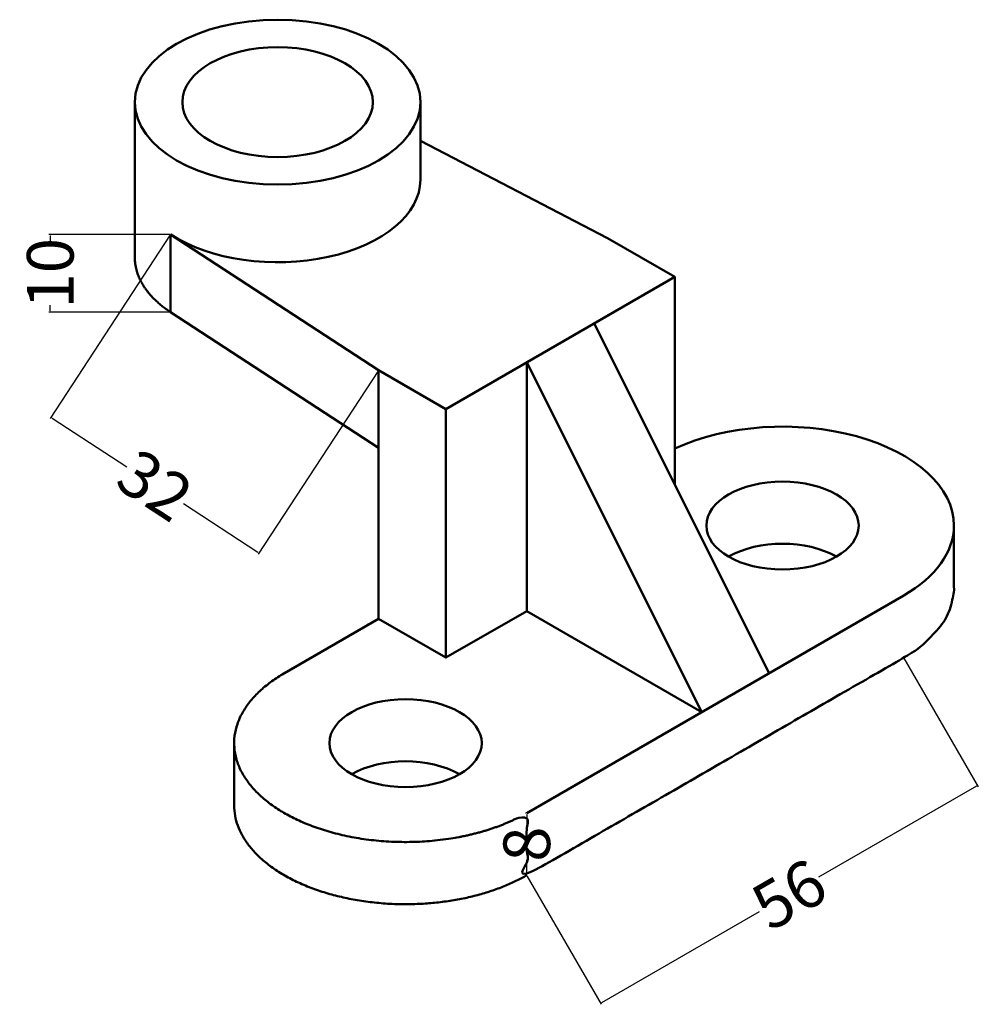
# Model space of a CAD drawing. Units: millimetres. Extents: x -12 to 111, y 15 to 142.
import ezdxf

# ---------------------------------------------------------------- set-up
doc = ezdxf.new("R2010")
doc.units = ezdxf.units.MM
doc.header["$MEASUREMENT"] = 0
doc.layers.add('M-DIMS', color=2, linetype='Continuous', lineweight=25)
doc.layers.add('M-OUTL', color=7, linetype='Continuous', lineweight=50)
doc.styles.get("Standard").update_dxf_attribs({"font": 'arial.ttf'})
doc.dimstyles.get("Standard").update_dxf_attribs({"dimtxt": 6, "dimasz": 0.18, "dimexe": 0.18, "dimexo": 0.0625, "dimgap": 0.09, "dimtad": 0, "dimtoh": 1, "dimdec": 0, "dimzin": 0, "dimdsep": 46, "dimtxsty": 'Standard', "dimcen": 0.09, "dimadec": 0, "dimazin": 0, "dimtfac": 1, "dimtdec": 0, "dimtofl": 0, "dimtmove": 0, "dimatfit": 3, "dimfxl": 1, "dimtolj": 1, "dimtzin": 0, "dimarcsym": 0})

# ---------------------------------------------------------------- blocks, each defined once
blk = doc.blocks.new('*D1')
at = {"layer": 'Defpoints', "color": 0, "transparency": 16777216}
for p in [(101.81, 59.95), (111.31, 43.49), (53.32, 31.95)]:
    blk.add_point(p, dxfattribs=at)
at = {"layer": 'M-DIMS', "color": 0, "lineweight": -2, "transparency": 16777216}
for p, q in [((101.84, 59.89), (111.4, 43.34)), ((111.16, 43.4), (90.86, 31.69)), ((53.35, 31.89), (62.91, 15.34)), ((62.97, 15.58), (83.27, 27.3))]:
    blk.add_line(p, q, dxfattribs=at)
at = {"layer": 'M-DIMS', "color": 0, "transparency": 16777216}
for points in [[(111.14, 43.43), (111.17, 43.38), (111.31, 43.49)], [(62.96, 15.61), (62.99, 15.56), (62.82, 15.49)]]:
    blk.add_solid(points, dxfattribs=at)
at = {"layer": 'M-DIMS', "color": 0, "transparency": 16777216, "insert": (87.06, 29.49), "char_height": 6, "attachment_point": 5, "rotation": 30}
blk.add_mtext('\\A1;56', dxfattribs=at)
blk = doc.blocks.new('*D2')
at = {"layer": 'Defpoints', "color": 0, "transparency": 16777216}
for p in [(7.51, 114.42), (34.26, 96.95), (18.89, 73.4)]:
    blk.add_point(p, dxfattribs=at)
at = {"layer": 'M-DIMS', "color": 0, "lineweight": -2, "transparency": 16777216}
for p, q in [((7.47, 114.37), (-7.97, 90.73)), ((34.23, 96.9), (18.79, 73.25)), ((-7.72, 90.78), (1.86, 84.52)), ((18.74, 73.5), (9.15, 79.76))]:
    blk.add_line(p, q, dxfattribs=at)
at = {"layer": 'M-DIMS', "color": 0, "transparency": 16777216}
for points in [[(-7.7, 90.81), (-7.73, 90.76), (-7.87, 90.88)], [(18.75, 73.53), (18.72, 73.48), (18.89, 73.4)]]:
    blk.add_solid(points, dxfattribs=at)
at = {"layer": 'M-DIMS', "color": 0, "transparency": 16777216, "insert": (5.51, 82.14), "char_height": 6, "attachment_point": 5, "rotation": 326.8489}
blk.add_mtext('\\A1;32', dxfattribs=at)
blk = doc.blocks.new('*D3')
at = {"layer": 'Defpoints', "color": 0, "transparency": 16777216}
for p in [(7.51, 114.42), (-7.97, 104.42), (7.51, 104.42)]:
    blk.add_point(p, dxfattribs=at)
at = {"layer": 'M-DIMS', "color": 0, "lineweight": -2, "transparency": 16777216}
for p, q in [((7.45, 114.42), (-8.15, 114.42)), ((-7.97, 114.24), (-7.97, 113.52)), ((-7.97, 104.6), (-7.97, 105.33)), ((7.45, 104.42), (-8.15, 104.42))]:
    blk.add_line(p, q, dxfattribs=at)
at = {"layer": 'M-DIMS', "color": 0, "transparency": 16777216}
for points in [[(-8, 114.24), (-7.94, 114.24), (-7.97, 114.42)], [(-8, 104.6), (-7.94, 104.6), (-7.97, 104.42)]]:
    blk.add_solid(points, dxfattribs=at)
at = {"layer": 'M-DIMS', "color": 0, "transparency": 16777216, "insert": (-7.97, 109.42), "char_height": 6, "attachment_point": 5, "rotation": 90}
blk.add_mtext('\\A1;10', dxfattribs=at)
blk = doc.blocks.new('*D4')
at = {"layer": 'Defpoints', "color": 0, "transparency": 16777216}
for p in [(53.32, 39.95), (53.32, 31.95), (53.32, 31.95)]:
    blk.add_point(p, dxfattribs=at)
at = {"layer": 'M-DIMS', "color": 0, "lineweight": -2, "transparency": 16777216}
for p, q in [((53.25, 39.95), (53.14, 39.95)), ((53.32, 39.77), (53.32, 38.01)), ((53.32, 32.13), (53.32, 33.88)), ((53.25, 31.95), (53.14, 31.95))]:
    blk.add_line(p, q, dxfattribs=at)
at = {"layer": 'M-DIMS', "color": 0, "transparency": 16777216}
for points in [[(53.29, 39.77), (53.35, 39.77), (53.32, 39.95)], [(53.29, 32.13), (53.35, 32.13), (53.32, 31.95)]]:
    blk.add_solid(points, dxfattribs=at)
at = {"layer": 'M-DIMS', "color": 0, "transparency": 16777216, "insert": (53.32, 35.95), "char_height": 6, "attachment_point": 5, "rotation": 90}
blk.add_mtext('\\A1;8', dxfattribs=at)

msp = doc.modelspace()

# ---------------------------------------------------------------- linework, layer by layer
at = {"layer": 'M-OUTL'}
for p, q in [((39.64, 121.45), (39.64, 131.45)), ((72.37, 82.18), (72.37, 108.95)), ((61.98, 102.95), (84.49, 57.95)), ((57.65, 100.45), (57.65, 100.45)), ((34.26, 96.95), (42.92, 91.95))]:
    msp.add_line(p, q, dxfattribs=at)
for points in [[(42.92, 59.95), (42.92, 91.95), (72.37, 108.95), (63.71, 113.95), (39.64, 126.45)], [(34.26, 96.95), (34.26, 64.95), (42.92, 59.95), (53.32, 65.95)], [(101.81, 67.95), (53.32, 39.95)], [(22.14, 57.95), (34.26, 64.95)]]:
    msp.add_lwpolyline(points, dxfattribs=at)
for points in [[(7.51, 114.42), (7.51, 104.42), (34.26, 86.95), (34.26, 96.95)], [(53.32, 65.95), (53.32, 97.95), (75.83, 52.95)]]:
    msp.add_lwpolyline(points, close=True, dxfattribs=at)
for centre, major_axis in [((21.27, 131.45), (-18.37, 0)), ((21.27, 131.45), (-12.25, 0)), ((86.22, 76.95), (-9.8, 0)), ((37.73, 48.95), (-9.8, 0))]:
    msp.add_ellipse(centre, major_axis=major_axis, ratio=0.57735, dxfattribs=at)
for centre, major_axis, start_param, end_param in [((21.27, 121.45), (18.37, 0), 3.867437, 6.283185), ((86.22, 76.95), (22.05, 0), 0, 2.25047), ((86.22, 76.95), (22.05, 0), 5.497787, 6.283185), ((86.22, 68.95), (-9.8, 0), 3.926991, 5.497787), ((37.73, 40.95), (-9.8, 0), 3.926991, 5.497787)]:
    msp.add_ellipse(centre, major_axis=major_axis, ratio=0.57735, start_param=start_param, end_param=end_param, dxfattribs=at)
for points, weights, knots in [([(2.9, 131.45), (2.9, 121.45), (2.9, 111.45), (2.9, 107.43), (7.51, 104.42)], [1, 1, 1, 0.935214346655, 1], [0, 0, 0, 1, 1, 1.723865, 1.723865, 1.723865]), ([(29.07, 61.95), (31.67, 63.45), (34.26, 64.95), (28.2, 61.45), (22.14, 57.95), (6.55, 48.95), (22.14, 39.95), (37.73, 30.95), (53.32, 39.95), (53.32, 35.95), (53.32, 31.95), (77.56, 45.95), (101.81, 59.95), (108.27, 63.68), (108.27, 68.95), (108.27, 72.95), (108.27, 76.95)], [1, 1, 1, 1, 1, 0.707106781187, 1, 0.707106781187, 1, 1, 1, 1, 1, 0.923879532511, 1, 1, 1], [0, 0, 0, 1, 1, 2, 2, 3.570796, 3.570796, 5.141593, 5.141593, 6.141593, 6.141593, 7.141593, 7.141593, 7.926991, 7.926991, 8.926991, 8.926991, 8.926991]), ([(15.68, 48.95), (15.68, 44.95), (15.68, 40.95), (15.68, 32.44), (29.29, 29.19), (42.9, 25.93), (53.32, 31.95)], [1, 1, 1, 0.831469612303, 1, 0.831469612303, 1], [0, 0, 0, 1, 1, 2.178097, 2.178097, 3.356194, 3.356194, 3.356194])]:
    msp.add_rational_spline(points, weights, degree=2, knots=knots, dxfattribs=at)

# ---------------------------------------------------------------- dimensions: what is measured, and where the dimension line sits
at = {"layer": 'M-DIMS'}
for p1, p2, distance, picture, middle in [((7.51, 114.42), (7.51, 104.42), -15.48, '*D3', (-7.97, 109.42)), ((7.51, 114.42), (34.26, 96.95), -28.12, '*D2', (5.51, 82.14)), ((53.32, 31.95), (101.81, 59.95), -19, '*D1', (87.06, 29.49)), ((53.32, 39.95), (53.32, 31.95), 0, '*D4', (53.32, 35.95))]:
    dim = msp.add_aligned_dim(p1=p1, p2=p2, distance=distance, dimstyle='Standard', override={"dimclrd": 0, "dimclre": 0, "dimclrt": 0}, dxfattribs=at)
    dim.commit()
    dim.dimension.update_dxf_attribs({"geometry": picture, "text_midpoint": middle})

doc.saveas('drawing.dxf')
